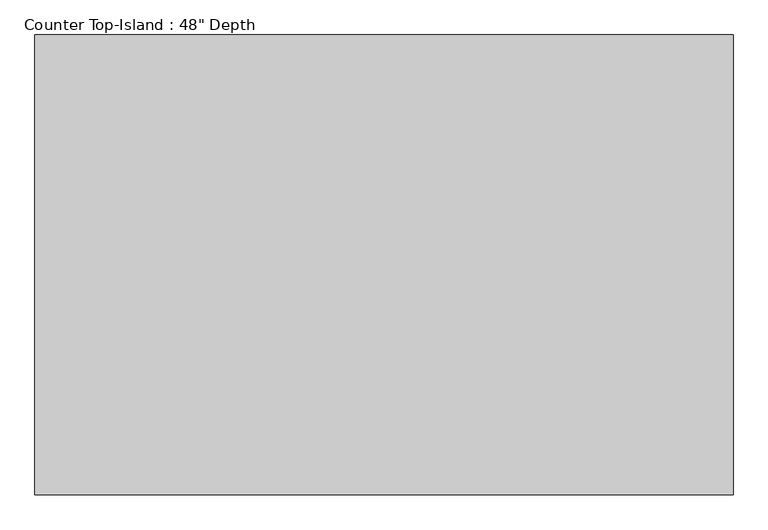
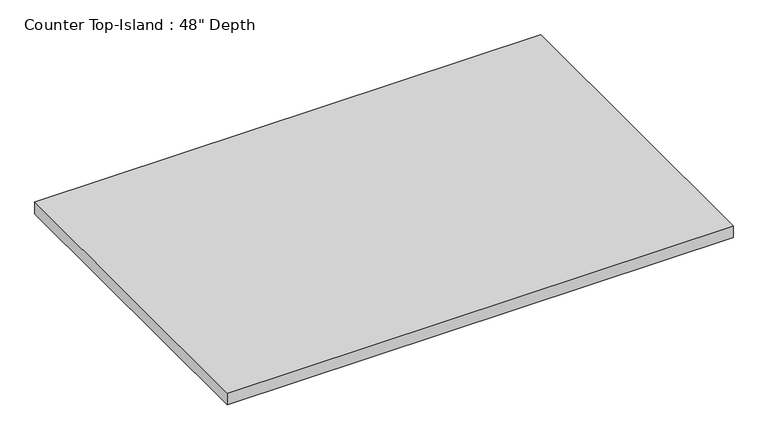
"""IFC4 building model written with IfcOpenShell, lengths in millimetres: furniture geometry."""

from ifc_helpers import new_model, si_unit, frame, origin, place, context, project, spatial, polyline, outline, extrude, source, transform, mapped, element, save


def furniture_ac307b45(model_context):
    return source(origin(), model_context, "Body", "SweptSolid", [
        extrude(outline(polyline([(342.5877049, 25.4), (342.5877049, -991.3330544), (-1200.4622951, -991.3330544), (-1200.4622951, 25.4), (342.5877049, 25.4)])), frame((0.0, 0.0, 876.3), z_axis=(0.0, 0.0, 1.0), x_axis=(1.0, 0.0, 0.0)), (0.0, 0.0, 1.0), 38.1),
    ])


if __name__ == "__main__":
    model = new_model("IFC4")
    model_context = context("Model", 3, world=origin())
    ifc_project = project(units=[si_unit("LENGTHUNIT", "METRE", prefix="MILLI")], contexts=[model_context])
    site = spatial("IfcSite", under=ifc_project)
    building = spatial("IfcBuilding", under=site)
    placement = place(None, origin())
    furniture_shape = furniture_ac307b45(model_context)
    element("IfcFurniture", 1, ObjectType="Counter Top-Island : 48\" Depth", at=placement, inside=building, context=model_context, shape_type="MappedRepresentation", body=[
        mapped(furniture_shape, transform((0.0, 0.0, 0.0), x_axis=(1.0, 0.0, 0.0), y_axis=(0.0, 1.0, 0.0), z_axis=(0.0, 0.0, 1.0))),
    ])
    save(model, "model.ifc")

# Revit data of these elements
# Type "Counter Top-Island : 48\" Depth"
#   Assembly Code = "C1030400"
#   Counter Thickness = 0' - 1 1/2"
#   Depth [instance default] = 4' - 2"
#   Height = 3' - 0"
#   Length [instance default] = 8' - 0"
#   Counter Top Material = none
#   Default Elevation = 0
# Element 1 (IfcFurniture, "Counter Top-Island : 48\" Depth")
#   Depth = 3' - 4.02886"
#   Length = 5' - 0 3/4"
#   Materials on its faces: "Counter Top"
# Materials
#   "Counter Top": class "Wood", colour RGB 226 177 128, transparency 0
